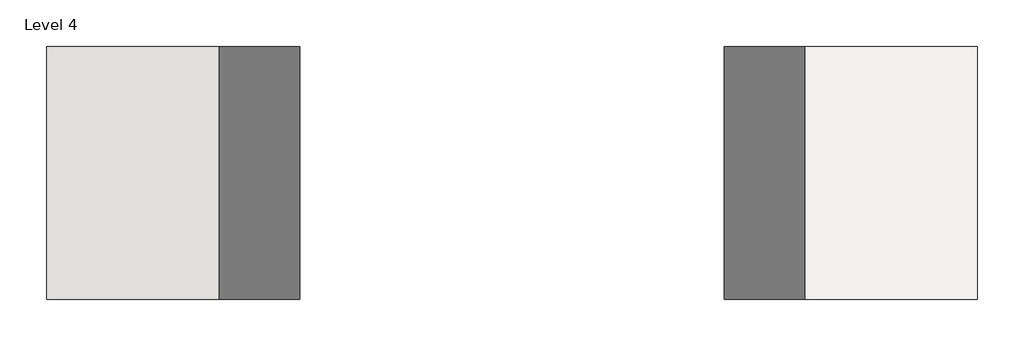
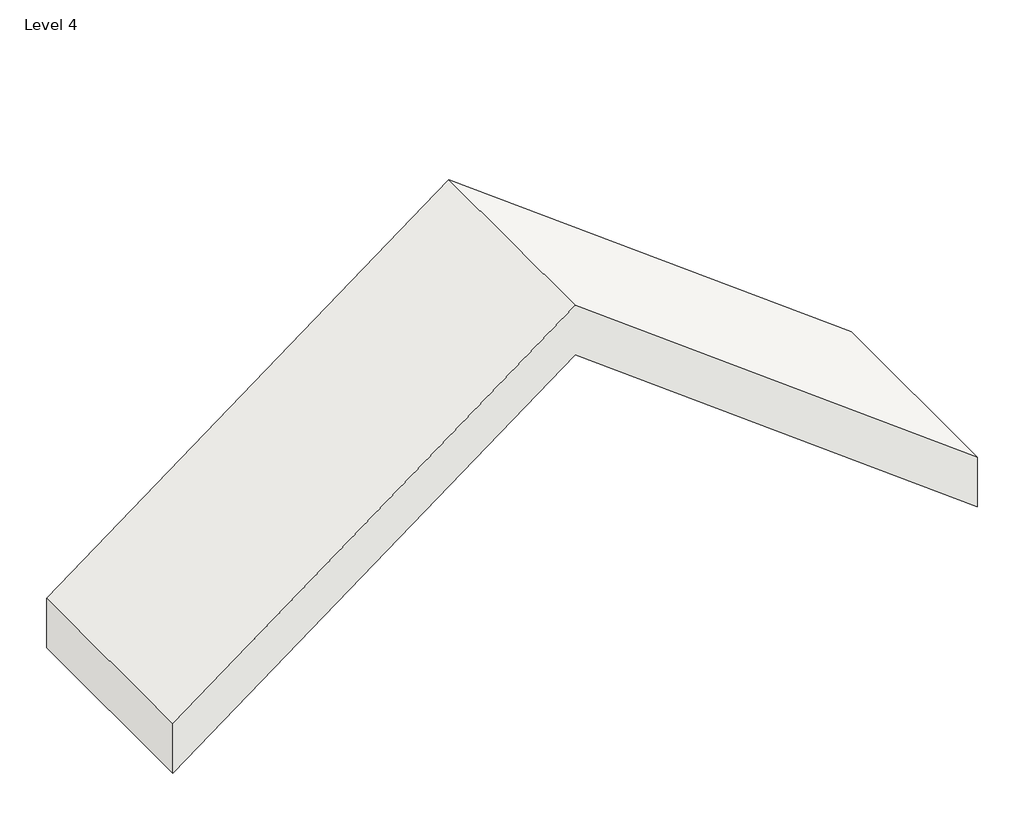
# One storey: 1 roof.
"""IFC4 building model written with IfcOpenShell, lengths in millimetres."""

from ifc_helpers import new_model, si_unit, frame, origin, place, context, project, spatial, polyline, outline, extrude, element, save

model = new_model("IFC4")

# Units and contexts
model_context = context("Model", 3, world=origin())
ifc_project = project(units=[si_unit("LENGTHUNIT", "METRE", prefix="MILLI")], contexts=[model_context])

# Site, building, storey
site = spatial("IfcSite", under=ifc_project)
building = spatial("IfcBuilding", under=site)
storey = spatial("IfcBuildingStorey", under=building, Name="Level 4", Elevation=9144.0)

# Roof
placement = place(None, origin())
element("IfcRoof", 1, ObjectType="Generic - 12\"", at=placement, inside=storey, context=model_context, shape_type="SweptSolid", body=[
    extrude(outline(polyline([(9525.0, -3141.477979), (11729.8892936, -6081.3303705), (9525.0, -9021.182762), (9144.0, -9021.182762), (11348.8892936, -6081.3303705), (9144.0, -3141.477979), (9525.0, -3141.477979)])), frame((0.0, -11959.0047424, 0.0), z_axis=(0.0, 1.0, 0.0), x_axis=(0.0, 0.0, 1.0)), (0.0, 0.0, 1.0), 1600.2),
])

save(model, "model.ifc")

# Revit data of these elements
# Type "Generic - 12\""
#   Assembly Code = "B1020"
#   Layers, outside or top first: 1' - 0" no material (function 1)
# Element 1 (IfcRoof, "Generic - 12\"")
#   built-in parameter 1001705 = 38.4839 (stored number, unit not read)
#   built-in parameter 1001710 = 33615
#   Phase Created = New Construction
#   Materials on its faces: "Default Roof"
# Materials
#   "Default Roof": colour RGB 88 101 114, transparency 0, Cost = 0
